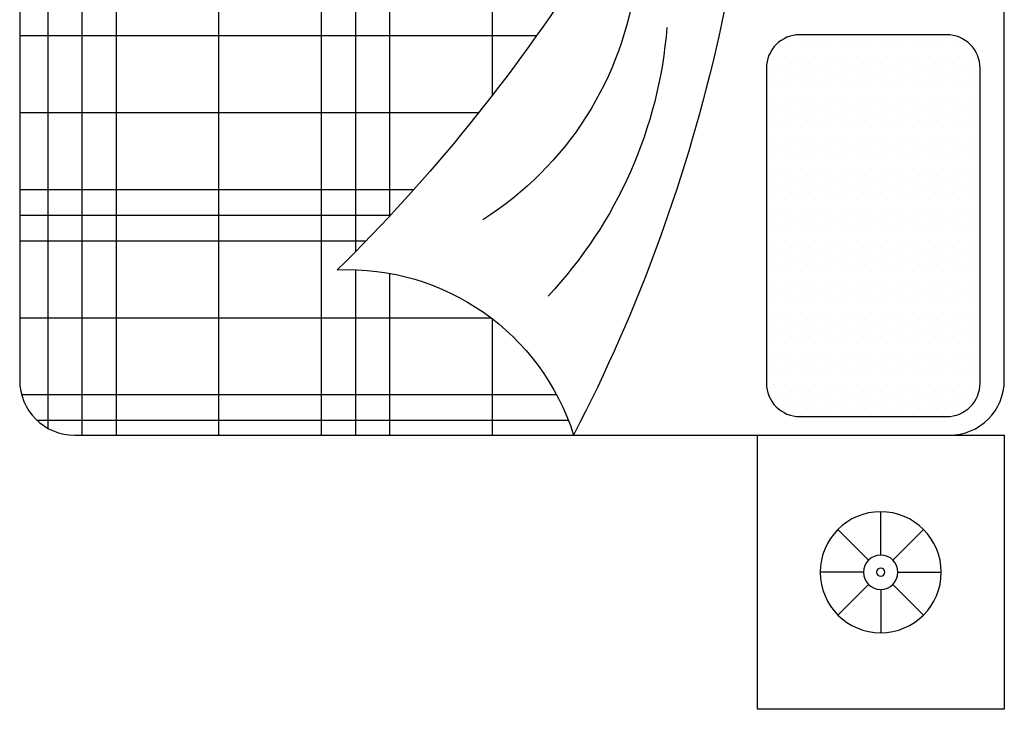
# Model space of a CAD drawing. Units: inches. Extents: x 528 to 2520, y -151 to 1354.
# Tile 38 of 41: x 2385 to 2440, y 731 to 770. Entities that reach past the tile are written whole.
import ezdxf

# ---------------------------------------------------------------- set-up
doc = ezdxf.new("R2010")
doc.units = ezdxf.units.IN
doc.header["$MEASUREMENT"] = 0
doc.layers.add('A-FURN', color=8, linetype='Continuous', lineweight=18)
doc.layers.add('BLOCK', color=6, linetype='Continuous')

# ---------------------------------------------------------------- blocks, each defined once
blk = doc.blocks.new('*X15')
at = {"color": 0}
for p, q in [((276.598, 451.25), (280.51, 451.25)), ((275.455, 450.625), (280.51, 450.625)), ((274.411, 450), (280.51, 450)), ((265.51, 448.125), (267.634, 448.125)), ((271.723, 448.125), (280.51, 448.125)), ((265.51, 446.25), (268.465, 446.25)), ((269.519, 446.25), (280.51, 446.25)), ((265.51, 445.625), (268.531, 445.625)), ((268.866, 445.625), (280.51, 445.625)), ((265.51, 445), (280.51, 445)), ((265.51, 443.125), (280.51, 443.125)), ((265.51, 441.25), (280.51, 441.25)), ((265.51, 440.625), (280.51, 440.625)), ((265.634, 440), (280.386, 440))]:
    blk.add_line(p, q, dxfattribs=at)
blk = doc.blocks.new('*X16')
at = {"color": 0}
for p, q in [((280.312, 439.886), (280.312, 452.896)), ((278.906, 439.482), (278.906, 452.338)), ((277.5, 439.482), (277.5, 451.702)), ((277.031, 439.482), (277.031, 451.471)), ((276.562, 439.482), (276.562, 451.231)), ((275.156, 439.482), (275.156, 450.451)), ((265.781, 439.797), (265.781, 449.511)), ((273.75, 439.482), (273.75, 449.576)), ((266.25, 439.517), (266.25, 449.296)), ((273.281, 439.482), (273.281, 449.261)), ((272.812, 439.482), (272.812, 448.934)), ((267.656, 439.482), (267.656, 448.095)), ((271.406, 439.482), (271.406, 447.876)), ((270, 439.482), (270, 446.689)), ((269.531, 439.482), (269.531, 446.262)), ((269.062, 439.482), (269.062, 445.817))]:
    blk.add_line(p, q, dxfattribs=at)
blk = doc.blocks.new('*X17')
at = {"color": 0}
for p, q in [((266.4375, 457.03125), (266.4375, 457.03125)), ((266.8125, 457.03125), (266.8125, 457.03125)), ((267.1875, 457.03125), (267.1875, 457.03125)), ((267.5625, 457.03125), (267.5625, 457.03125)), ((267.9375, 457.03125), (267.9375, 457.03125)), ((268.3125, 457.03125), (268.3125, 457.03125)), ((268.6875, 457.03125), (268.6875, 457.03125)), ((269.0625, 457.03125), (269.0625, 457.03125)), ((269.4375, 457.03125), (269.4375, 457.03125)), ((269.8125, 457.03125), (269.8125, 457.03125)), ((270.1875, 457.03125), (270.1875, 457.03125)), ((270.5625, 457.03125), (270.5625, 457.03125)), ((270.9375, 457.03125), (270.9375, 457.03125)), ((271.3125, 457.03125), (271.3125, 457.03125)), ((271.6875, 457.03125), (271.6875, 457.03125)), ((272.0625, 457.03125), (272.0625, 457.03125)), ((266.0625, 456.84375), (266.0625, 456.84375)), ((266.25, 456.9375), (266.25, 456.9375)), ((266.4375, 456.84375), (266.4375, 456.84375)), ((266.625, 456.9375), (266.625, 456.9375)), ((266.8125, 456.84375), (266.8125, 456.84375)), ((267, 456.9375), (267, 456.9375)), ((267.1875, 456.84375), (267.1875, 456.84375)), ((267.375, 456.9375), (267.375, 456.9375)), ((267.5625, 456.84375), (267.5625, 456.84375)), ((267.75, 456.9375), (267.75, 456.9375)), ((267.9375, 456.84375), (267.9375, 456.84375)), ((268.125, 456.9375), (268.125, 456.9375)), ((268.3125, 456.84375), (268.3125, 456.84375)), ((268.5, 456.9375), (268.5, 456.9375)), ((268.6875, 456.84375), (268.6875, 456.84375)), ((268.875, 456.9375), (268.875, 456.9375)), ((269.0625, 456.84375), (269.0625, 456.84375)), ((269.25, 456.9375), (269.25, 456.9375)), ((269.4375, 456.84375), (269.4375, 456.84375)), ((269.625, 456.9375), (269.625, 456.9375)), ((269.8125, 456.84375), (269.8125, 456.84375)), ((270, 456.9375), (270, 456.9375)), ((270.1875, 456.84375), (270.1875, 456.84375)), ((270.375, 456.9375), (270.375, 456.9375)), ((270.5625, 456.84375), (270.5625, 456.84375)), ((270.75, 456.9375), (270.75, 456.9375)), ((270.9375, 456.84375), (270.9375, 456.84375)), ((271.125, 456.9375), (271.125, 456.9375)), ((271.3125, 456.84375), (271.3125, 456.84375)), ((271.5, 456.9375), (271.5, 456.9375)), ((271.6875, 456.84375), (271.6875, 456.84375)), ((271.875, 456.9375), (271.875, 456.9375)), ((272.0625, 456.84375), (272.0625, 456.84375)), ((272.25, 456.9375), (272.25, 456.9375)), ((272.4375, 456.84375), (272.4375, 456.84375)), ((266.25, 456.75), (266.25, 456.75)), ((266.625, 456.75), (266.625, 456.75)), ((267, 456.75), (267, 456.75)), ((267.375, 456.75), (267.375, 456.75)), ((267.75, 456.75), (267.75, 456.75)), ((268.125, 456.75), (268.125, 456.75)), ((268.5, 456.75), (268.5, 456.75)), ((268.875, 456.75), (268.875, 456.75)), ((269.25, 456.75), (269.25, 456.75)), ((269.625, 456.75), (269.625, 456.75)), ((270, 456.75), (270, 456.75)), ((270.375, 456.75), (270.375, 456.75)), ((270.75, 456.75), (270.75, 456.75)), ((271.125, 456.75), (271.125, 456.75)), ((271.5, 456.75), (271.5, 456.75)), ((271.875, 456.75), (271.875, 456.75)), ((272.25, 456.75), (272.25, 456.75)), ((272.625, 456.75), (272.625, 456.75)), ((265.875, 456.5625), (265.875, 456.5625)), ((266.0625, 456.65625), (266.0625, 456.65625)), ((266.25, 456.5625), (266.25, 456.5625)), ((266.4375, 456.65625), (266.4375, 456.65625)), ((266.625, 456.5625), (266.625, 456.5625)), ((266.8125, 456.65625), (266.8125, 456.65625)), ((267, 456.5625), (267, 456.5625)), ((267.1875, 456.65625), (267.1875, 456.65625)), ((267.375, 456.5625), (267.375, 456.5625)), ((267.5625, 456.65625), (267.5625, 456.65625)), ((267.75, 456.5625), (267.75, 456.5625)), ((267.9375, 456.65625), (267.9375, 456.65625)), ((268.125, 456.5625), (268.125, 456.5625)), ((268.3125, 456.65625), (268.3125, 456.65625)), ((268.5, 456.5625), (268.5, 456.5625)), ((268.6875, 456.65625), (268.6875, 456.65625)), ((268.875, 456.5625), (268.875, 456.5625)), ((269.0625, 456.65625), (269.0625, 456.65625)), ((269.25, 456.5625), (269.25, 456.5625)), ((269.4375, 456.65625), (269.4375, 456.65625)), ((269.625, 456.5625), (269.625, 456.5625)), ((269.8125, 456.65625), (269.8125, 456.65625)), ((270, 456.5625), (270, 456.5625)), ((270.1875, 456.65625), (270.1875, 456.65625)), ((270.375, 456.5625), (270.375, 456.5625)), ((270.5625, 456.65625), (270.5625, 456.65625)), ((270.75, 456.5625), (270.75, 456.5625)), ((270.9375, 456.65625), (270.9375, 456.65625)), ((271.125, 456.5625), (271.125, 456.5625)), ((271.3125, 456.65625), (271.3125, 456.65625)), ((271.5, 456.5625), (271.5, 456.5625)), ((271.6875, 456.65625), (271.6875, 456.65625)), ((271.875, 456.5625), (271.875, 456.5625)), ((272.0625, 456.65625), (272.0625, 456.65625)), ((272.25, 456.5625), (272.25, 456.5625)), ((272.4375, 456.65625), (272.4375, 456.65625)), ((272.625, 456.5625), (272.625, 456.5625)), ((265.875, 456.375), (265.875, 456.375)), ((266.0625, 456.46875), (266.0625, 456.46875)), ((266.25, 456.375), (266.25, 456.375)), ((266.4375, 456.46875), (266.4375, 456.46875)), ((266.625, 456.375), (266.625, 456.375)), ((266.8125, 456.46875), (266.8125, 456.46875)), ((267, 456.375), (267, 456.375)), ((267.1875, 456.46875), (267.1875, 456.46875)), ((267.375, 456.375), (267.375, 456.375)), ((267.5625, 456.46875), (267.5625, 456.46875)), ((267.75, 456.375), (267.75, 456.375)), ((267.9375, 456.46875), (267.9375, 456.46875)), ((268.125, 456.375), (268.125, 456.375)), ((268.3125, 456.46875), (268.3125, 456.46875)), ((268.5, 456.375), (268.5, 456.375)), ((268.6875, 456.46875), (268.6875, 456.46875)), ((268.875, 456.375), (268.875, 456.375)), ((269.0625, 456.46875), (269.0625, 456.46875)), ((269.25, 456.375), (269.25, 456.375)), ((269.4375, 456.46875), (269.4375, 456.46875)), ((269.625, 456.375), (269.625, 456.375)), ((269.8125, 456.46875), (269.8125, 456.46875)), ((270, 456.375), (270, 456.375)), ((270.1875, 456.46875), (270.1875, 456.46875)), ((270.375, 456.375), (270.375, 456.375)), ((270.5625, 456.46875), (270.5625, 456.46875)), ((270.75, 456.375), (270.75, 456.375)), ((270.9375, 456.46875), (270.9375, 456.46875)), ((271.125, 456.375), (271.125, 456.375)), ((271.3125, 456.46875), (271.3125, 456.46875)), ((271.5, 456.375), (271.5, 456.375)), ((271.6875, 456.46875), (271.6875, 456.46875)), ((271.875, 456.375), (271.875, 456.375)), ((272.0625, 456.46875), (272.0625, 456.46875)), ((272.25, 456.375), (272.25, 456.375)), ((272.4375, 456.46875), (272.4375, 456.46875)), ((272.625, 456.375), (272.625, 456.375)), ((272.8125, 456.46875), (272.8125, 456.46875)), ((265.875, 456.1875), (265.875, 456.1875)), ((266.0625, 456.28125), (266.0625, 456.28125)), ((266.25, 456.1875), (266.25, 456.1875)), ((266.4375, 456.28125), (266.4375, 456.28125)), ((266.625, 456.1875), (266.625, 456.1875)), ((266.8125, 456.28125), (266.8125, 456.28125)), ((267, 456.1875), (267, 456.1875)), ((267.1875, 456.28125), (267.1875, 456.28125)), ((267.375, 456.1875), (267.375, 456.1875)), ((267.5625, 456.28125), (267.5625, 456.28125)), ((267.75, 456.1875), (267.75, 456.1875)), ((267.9375, 456.28125), (267.9375, 456.28125)), ((268.125, 456.1875), (268.125, 456.1875)), ((268.3125, 456.28125), (268.3125, 456.28125)), ((268.5, 456.1875), (268.5, 456.1875)), ((268.6875, 456.28125), (268.6875, 456.28125)), ((268.875, 456.1875), (268.875, 456.1875)), ((269.0625, 456.28125), (269.0625, 456.28125)), ((269.25, 456.1875), (269.25, 456.1875)), ((269.4375, 456.28125), (269.4375, 456.28125)), ((269.625, 456.1875), (269.625, 456.1875)), ((269.8125, 456.28125), (269.8125, 456.28125)), ((270, 456.1875), (270, 456.1875)), ((270.1875, 456.28125), (270.1875, 456.28125)), ((270.375, 456.1875), (270.375, 456.1875)), ((270.5625, 456.28125), (270.5625, 456.28125)), ((270.75, 456.1875), (270.75, 456.1875)), ((270.9375, 456.28125), (270.9375, 456.28125)), ((271.125, 456.1875), (271.125, 456.1875)), ((271.3125, 456.28125), (271.3125, 456.28125)), ((271.5, 456.1875), (271.5, 456.1875)), ((271.6875, 456.28125), (271.6875, 456.28125)), ((271.875, 456.1875), (271.875, 456.1875)), ((272.0625, 456.28125), (272.0625, 456.28125)), ((272.25, 456.1875), (272.25, 456.1875)), ((272.4375, 456.28125), (272.4375, 456.28125)), ((272.625, 456.1875), (272.625, 456.1875)), ((272.8125, 456.28125), (272.8125, 456.28125)), ((265.875, 456), (265.875, 456)), ((266.0625, 456.09375), (266.0625, 456.09375)), ((266.25, 456), (266.25, 456)), ((266.4375, 456.09375), (266.4375, 456.09375)), ((266.625, 456), (266.625, 456)), ((266.8125, 456.09375), (266.8125, 456.09375)), ((267, 456), (267, 456)), ((267.1875, 456.09375), (267.1875, 456.09375)), ((267.375, 456), (267.375, 456)), ((267.5625, 456.09375), (267.5625, 456.09375)), ((267.75, 456), (267.75, 456)), ((267.9375, 456.09375), (267.9375, 456.09375)), ((268.125, 456), (268.125, 456)), ((268.3125, 456.09375), (268.3125, 456.09375)), ((268.5, 456), (268.5, 456)), ((268.6875, 456.09375), (268.6875, 456.09375)), ((268.875, 456), (268.875, 456)), ((269.0625, 456.09375), (269.0625, 456.09375)), ((269.25, 456), (269.25, 456)), ((269.4375, 456.09375), (269.4375, 456.09375)), ((269.625, 456), (269.625, 456)), ((269.8125, 456.09375), (269.8125, 456.09375)), ((270, 456), (270, 456)), ((270.1875, 456.09375), (270.1875, 456.09375)), ((270.375, 456), (270.375, 456)), ((270.5625, 456.09375), (270.5625, 456.09375)), ((270.75, 456), (270.75, 456)), ((270.9375, 456.09375), (270.9375, 456.09375)), ((271.125, 456), (271.125, 456)), ((271.3125, 456.09375), (271.3125, 456.09375)), ((271.5, 456), (271.5, 456)), ((271.6875, 456.09375), (271.6875, 456.09375)), ((271.875, 456), (271.875, 456)), ((272.0625, 456.09375), (272.0625, 456.09375)), ((272.25, 456), (272.25, 456)), ((272.4375, 456.09375), (272.4375, 456.09375)), ((272.625, 456), (272.625, 456)), ((272.8125, 456.09375), (272.8125, 456.09375)), ((265.875, 455.8125), (265.875, 455.8125)), ((266.0625, 455.90625), (266.0625, 455.90625)), ((266.25, 455.8125), (266.25, 455.8125)), ((266.4375, 455.90625), (266.4375, 455.90625)), ((266.625, 455.8125), (266.625, 455.8125)), ((266.8125, 455.90625), (266.8125, 455.90625)), ((267, 455.8125), (267, 455.8125)), ((267.1875, 455.90625), (267.1875, 455.90625)), ((267.375, 455.8125), (267.375, 455.8125)), ((267.5625, 455.90625), (267.5625, 455.90625)), ((267.75, 455.8125), (267.75, 455.8125)), ((267.9375, 455.90625), (267.9375, 455.90625)), ((268.125, 455.8125), (268.125, 455.8125)), ((268.3125, 455.90625), (268.3125, 455.90625)), ((268.5, 455.8125), (268.5, 455.8125)), ((268.6875, 455.90625), (268.6875, 455.90625)), ((268.875, 455.8125), (268.875, 455.8125)), ((269.0625, 455.90625), (269.0625, 455.90625)), ((269.25, 455.8125), (269.25, 455.8125)), ((269.4375, 455.90625), (269.4375, 455.90625)), ((269.625, 455.8125), (269.625, 455.8125)), ((269.8125, 455.90625), (269.8125, 455.90625)), ((270, 455.8125), (270, 455.8125)), ((270.1875, 455.90625), (270.1875, 455.90625)), ((270.375, 455.8125), (270.375, 455.8125)), ((270.5625, 455.90625), (270.5625, 455.90625)), ((270.75, 455.8125), (270.75, 455.8125)), ((270.9375, 455.90625), (270.9375, 455.90625)), ((271.125, 455.8125), (271.125, 455.8125)), ((271.3125, 455.90625), (271.3125, 455.90625)), ((271.5, 455.8125), (271.5, 455.8125)), ((271.6875, 455.90625), (271.6875, 455.90625)), ((271.875, 455.8125), (271.875, 455.8125)), ((272.0625, 455.90625), (272.0625, 455.90625)), ((272.25, 455.8125), (272.25, 455.8125)), ((272.4375, 455.90625), (272.4375, 455.90625)), ((272.625, 455.8125), (272.625, 455.8125)), ((272.8125, 455.90625), (272.8125, 455.90625)), ((265.875, 455.625), (265.875, 455.625)), ((266.0625, 455.71875), (266.0625, 455.71875)), ((266.25, 455.625), (266.25, 455.625)), ((266.4375, 455.71875), (266.4375, 455.71875)), ((266.625, 455.625), (266.625, 455.625)), ((266.8125, 455.71875), (266.8125, 455.71875)), ((267, 455.625), (267, 455.625)), ((267.1875, 455.71875), (267.1875, 455.71875)), ((267.375, 455.625), (267.375, 455.625)), ((267.5625, 455.71875), (267.5625, 455.71875)), ((267.75, 455.625), (267.75, 455.625)), ((267.9375, 455.71875), (267.9375, 455.71875)), ((268.125, 455.625), (268.125, 455.625)), ((268.3125, 455.71875), (268.3125, 455.71875)), ((268.5, 455.625), (268.5, 455.625)), ((268.6875, 455.71875), (268.6875, 455.71875)), ((268.875, 455.625), (268.875, 455.625)), ((269.0625, 455.71875), (269.0625, 455.71875)), ((269.25, 455.625), (269.25, 455.625)), ((269.4375, 455.71875), (269.4375, 455.71875)), ((269.625, 455.625), (269.625, 455.625)), ((269.8125, 455.71875), (269.8125, 455.71875)), ((270, 455.625), (270, 455.625)), ((270.1875, 455.71875), (270.1875, 455.71875)), ((270.375, 455.625), (270.375, 455.625)), ((270.5625, 455.71875), (270.5625, 455.71875)), ((270.75, 455.625), (270.75, 455.625)), ((270.9375, 455.71875), (270.9375, 455.71875)), ((271.125, 455.625), (271.125, 455.625)), ((271.3125, 455.71875), (271.3125, 455.71875)), ((271.5, 455.625), (271.5, 455.625)), ((271.6875, 455.71875), (271.6875, 455.71875)), ((271.875, 455.625), (271.875, 455.625)), ((272.0625, 455.71875), (272.0625, 455.71875)), ((272.25, 455.625), (272.25, 455.625)), ((272.4375, 455.71875), (272.4375, 455.71875)), ((272.625, 455.625), (272.625, 455.625)), ((272.8125, 455.71875), (272.8125, 455.71875)), ((265.875, 455.4375), (265.875, 455.4375)), ((266.0625, 455.53125), (266.0625, 455.53125)), ((266.25, 455.4375), (266.25, 455.4375)), ((266.4375, 455.53125), (266.4375, 455.53125)), ((266.625, 455.4375), (266.625, 455.4375)), ((266.8125, 455.53125), (266.8125, 455.53125)), ((267, 455.4375), (267, 455.4375)), ((267.1875, 455.53125), (267.1875, 455.53125)), ((267.375, 455.4375), (267.375, 455.4375)), ((267.5625, 455.53125), (267.5625, 455.53125)), ((267.75, 455.4375), (267.75, 455.4375)), ((267.9375, 455.53125), (267.9375, 455.53125)), ((268.125, 455.4375), (268.125, 455.4375)), ((268.3125, 455.53125), (268.3125, 455.53125)), ((268.5, 455.4375), (268.5, 455.4375)), ((268.6875, 455.53125), (268.6875, 455.53125)), ((268.875, 455.4375), (268.875, 455.4375)), ((269.0625, 455.53125), (269.0625, 455.53125)), ((269.25, 455.4375), (269.25, 455.4375)), ((269.4375, 455.53125), (269.4375, 455.53125)), ((269.625, 455.4375), (269.625, 455.4375)), ((269.8125, 455.53125), (269.8125, 455.53125)), ((270, 455.4375), (270, 455.4375)), ((270.1875, 455.53125), (270.1875, 455.53125)), ((270.375, 455.4375), (270.375, 455.4375)), ((270.5625, 455.53125), (270.5625, 455.53125)), ((270.75, 455.4375), (270.75, 455.4375)), ((270.9375, 455.53125), (270.9375, 455.53125)), ((271.125, 455.4375), (271.125, 455.4375)), ((271.3125, 455.53125), (271.3125, 455.53125)), ((271.5, 455.4375), (271.5, 455.4375)), ((271.6875, 455.53125), (271.6875, 455.53125)), ((271.875, 455.4375), (271.875, 455.4375)), ((272.0625, 455.53125), (272.0625, 455.53125)), ((272.25, 455.4375), (272.25, 455.4375)), ((272.4375, 455.53125), (272.4375, 455.53125)), ((272.625, 455.4375), (272.625, 455.4375)), ((272.8125, 455.53125), (272.8125, 455.53125)), ((265.875, 455.25), (265.875, 455.25)), ((266.0625, 455.34375), (266.0625, 455.34375)), ((266.25, 455.25), (266.25, 455.25)), ((266.4375, 455.34375), (266.4375, 455.34375)), ((266.625, 455.25), (266.625, 455.25)), ((266.8125, 455.34375), (266.8125, 455.34375)), ((267, 455.25), (267, 455.25)), ((267.1875, 455.34375), (267.1875, 455.34375)), ((267.375, 455.25), (267.375, 455.25)), ((267.5625, 455.34375), (267.5625, 455.34375)), ((267.75, 455.25), (267.75, 455.25)), ((267.9375, 455.34375), (267.9375, 455.34375)), ((268.125, 455.25), (268.125, 455.25)), ((268.3125, 455.34375), (268.3125, 455.34375)), ((268.5, 455.25), (268.5, 455.25)), ((268.6875, 455.34375), (268.6875, 455.34375)), ((268.875, 455.25), (268.875, 455.25)), ((269.0625, 455.34375), (269.0625, 455.34375)), ((269.25, 455.25), (269.25, 455.25)), ((269.4375, 455.34375), (269.4375, 455.34375)), ((269.625, 455.25), (269.625, 455.25)), ((269.8125, 455.34375), (269.8125, 455.34375)), ((270, 455.25), (270, 455.25)), ((270.1875, 455.34375), (270.1875, 455.34375)), ((270.375, 455.25), (270.375, 455.25)), ((270.5625, 455.34375), (270.5625, 455.34375)), ((270.75, 455.25), (270.75, 455.25)), ((270.9375, 455.34375), (270.9375, 455.34375)), ((271.125, 455.25), (271.125, 455.25)), ((271.3125, 455.34375), (271.3125, 455.34375)), ((271.5, 455.25), (271.5, 455.25)), ((271.6875, 455.34375), (271.6875, 455.34375)), ((271.875, 455.25), (271.875, 455.25)), ((272.0625, 455.34375), (272.0625, 455.34375)), ((272.25, 455.25), (272.25, 455.25)), ((272.4375, 455.34375), (272.4375, 455.34375)), ((272.625, 455.25), (272.625, 455.25)), ((272.8125, 455.34375), (272.8125, 455.34375)), ((265.875, 455.0625), (265.875, 455.0625)), ((266.0625, 455.15625), (266.0625, 455.15625)), ((266.25, 455.0625), (266.25, 455.0625)), ((266.4375, 455.15625), (266.4375, 455.15625)), ((266.625, 455.0625), (266.625, 455.0625)), ((266.8125, 455.15625), (266.8125, 455.15625)), ((267, 455.0625), (267, 455.0625)), ((267.1875, 455.15625), (267.1875, 455.15625)), ((267.375, 455.0625), (267.375, 455.0625)), ((267.5625, 455.15625), (267.5625, 455.15625)), ((267.75, 455.0625), (267.75, 455.0625)), ((267.9375, 455.15625), (267.9375, 455.15625)), ((268.125, 455.0625), (268.125, 455.0625)), ((268.3125, 455.15625), (268.3125, 455.15625)), ((268.5, 455.0625), (268.5, 455.0625)), ((268.6875, 455.15625), (268.6875, 455.15625)), ((268.875, 455.0625), (268.875, 455.0625)), ((269.0625, 455.15625), (269.0625, 455.15625)), ((269.25, 455.0625), (269.25, 455.0625)), ((269.4375, 455.15625), (269.4375, 455.15625)), ((269.625, 455.0625), (269.625, 455.0625)), ((269.8125, 455.15625), (269.8125, 455.15625)), ((270, 455.0625), (270, 455.0625)), ((270.1875, 455.15625), (270.1875, 455.15625)), ((270.375, 455.0625), (270.375, 455.0625)), ((270.5625, 455.15625), (270.5625, 455.15625)), ((270.75, 455.0625), (270.75, 455.0625)), ((270.9375, 455.15625), (270.9375, 455.15625)), ((271.125, 455.0625), (271.125, 455.0625)), ((271.3125, 455.15625), (271.3125, 455.15625)), ((271.5, 455.0625), (271.5, 455.0625)), ((271.6875, 455.15625), (271.6875, 455.15625)), ((271.875, 455.0625), (271.875, 455.0625)), ((272.0625, 455.15625), (272.0625, 455.15625)), ((272.25, 455.0625), (272.25, 455.0625)), ((272.4375, 455.15625), (272.4375, 455.15625)), ((272.625, 455.0625), (272.625, 455.0625)), ((272.8125, 455.15625), (272.8125, 455.15625)), ((265.875, 454.875), (265.875, 454.875)), ((266.0625, 454.96875), (266.0625, 454.96875)), ((266.25, 454.875), (266.25, 454.875)), ((266.4375, 454.96875), (266.4375, 454.96875)), ((266.625, 454.875), (266.625, 454.875)), ((266.8125, 454.96875), (266.8125, 454.96875)), ((267, 454.875), (267, 454.875)), ((267.1875, 454.96875), (267.1875, 454.96875)), ((267.375, 454.875), (267.375, 454.875)), ((267.5625, 454.96875), (267.5625, 454.96875)), ((267.75, 454.875), (267.75, 454.875)), ((267.9375, 454.96875), (267.9375, 454.96875)), ((268.125, 454.875), (268.125, 454.875)), ((268.3125, 454.96875), (268.3125, 454.96875)), ((268.5, 454.875), (268.5, 454.875)), ((268.6875, 454.96875), (268.6875, 454.96875)), ((268.875, 454.875), (268.875, 454.875)), ((269.0625, 454.96875), (269.0625, 454.96875)), ((269.25, 454.875), (269.25, 454.875)), ((269.4375, 454.96875), (269.4375, 454.96875)), ((269.625, 454.875), (269.625, 454.875)), ((269.8125, 454.96875), (269.8125, 454.96875)), ((270, 454.875), (270, 454.875)), ((270.1875, 454.96875), (270.1875, 454.96875)), ((270.375, 454.875), (270.375, 454.875)), ((270.5625, 454.96875), (270.5625, 454.96875)), ((270.75, 454.875), (270.75, 454.875)), ((270.9375, 454.96875), (270.9375, 454.96875)), ((271.125, 454.875), (271.125, 454.875)), ((271.3125, 454.96875), (271.3125, 454.96875)), ((271.5, 454.875), (271.5, 454.875)), ((271.6875, 454.96875), (271.6875, 454.96875)), ((271.875, 454.875), (271.875, 454.875)), ((272.0625, 454.96875), (272.0625, 454.96875)), ((272.25, 454.875), (272.25, 454.875)), ((272.4375, 454.96875), (272.4375, 454.96875)), ((272.625, 454.875), (272.625, 454.875)), ((272.8125, 454.96875), (272.8125, 454.96875)), ((265.875, 454.6875), (265.875, 454.6875)), ((266.0625, 454.78125), (266.0625, 454.78125)), ((266.25, 454.6875), (266.25, 454.6875)), ((266.4375, 454.78125), (266.4375, 454.78125)), ((266.625, 454.6875), (266.625, 454.6875)), ((266.8125, 454.78125), (266.8125, 454.78125)), ((267, 454.6875), (267, 454.6875)), ((267.1875, 454.78125), (267.1875, 454.78125)), ((267.375, 454.6875), (267.375, 454.6875)), ((267.5625, 454.78125), (267.5625, 454.78125)), ((267.75, 454.6875), (267.75, 454.6875)), ((267.9375, 454.78125), (267.9375, 454.78125)), ((268.125, 454.6875), (268.125, 454.6875)), ((268.3125, 454.78125), (268.3125, 454.78125)), ((268.5, 454.6875), (268.5, 454.6875)), ((268.6875, 454.78125), (268.6875, 454.78125)), ((268.875, 454.6875), (268.875, 454.6875)), ((269.0625, 454.78125), (269.0625, 454.78125)), ((269.25, 454.6875), (269.25, 454.6875)), ((269.4375, 454.78125), (269.4375, 454.78125)), ((269.625, 454.6875), (269.625, 454.6875)), ((269.8125, 454.78125), (269.8125, 454.78125)), ((270, 454.6875), (270, 454.6875)), ((270.1875, 454.78125), (270.1875, 454.78125)), ((270.375, 454.6875), (270.375, 454.6875)), ((270.5625, 454.78125), (270.5625, 454.78125)), ((270.75, 454.6875), (270.75, 454.6875)), ((270.9375, 454.78125), (270.9375, 454.78125)), ((271.125, 454.6875), (271.125, 454.6875)), ((271.3125, 454.78125), (271.3125, 454.78125)), ((271.5, 454.6875), (271.5, 454.6875)), ((271.6875, 454.78125), (271.6875, 454.78125)), ((271.875, 454.6875), (271.875, 454.6875)), ((272.0625, 454.78125), (272.0625, 454.78125)), ((272.25, 454.6875), (272.25, 454.6875)), ((272.4375, 454.78125), (272.4375, 454.78125)), ((272.625, 454.6875), (272.625, 454.6875)), ((272.8125, 454.78125), (272.8125, 454.78125)), ((266.0625, 454.59375), (266.0625, 454.59375)), ((266.4375, 454.59375), (266.4375, 454.59375)), ((266.8125, 454.59375), (266.8125, 454.59375)), ((267.1875, 454.59375), (267.1875, 454.59375)), ((267.5625, 454.59375), (267.5625, 454.59375)), ((267.9375, 454.59375), (267.9375, 454.59375)), ((268.3125, 454.59375), (268.3125, 454.59375)), ((268.6875, 454.59375), (268.6875, 454.59375)), ((269.0625, 454.59375), (269.0625, 454.59375)), ((269.4375, 454.59375), (269.4375, 454.59375)), ((269.8125, 454.59375), (269.8125, 454.59375)), ((270.1875, 454.59375), (270.1875, 454.59375)), ((270.5625, 454.59375), (270.5625, 454.59375)), ((270.9375, 454.59375), (270.9375, 454.59375)), ((271.3125, 454.59375), (271.3125, 454.59375)), ((271.6875, 454.59375), (271.6875, 454.59375)), ((272.0625, 454.59375), (272.0625, 454.59375)), ((272.4375, 454.59375), (272.4375, 454.59375)), ((272.8125, 454.59375), (272.8125, 454.59375)), ((265.875, 454.5), (265.875, 454.5)), ((266.0625, 454.40625), (266.0625, 454.40625)), ((266.25, 454.5), (266.25, 454.5)), ((266.4375, 454.40625), (266.4375, 454.40625)), ((266.625, 454.5), (266.625, 454.5)), ((266.8125, 454.40625), (266.8125, 454.40625)), ((267, 454.5), (267, 454.5)), ((267.1875, 454.40625), (267.1875, 454.40625)), ((267.375, 454.5), (267.375, 454.5)), ((267.5625, 454.40625), (267.5625, 454.40625)), ((267.75, 454.5), (267.75, 454.5)), ((267.9375, 454.40625), (267.9375, 454.40625)), ((268.125, 454.5), (268.125, 454.5)), ((268.3125, 454.40625), (268.3125, 454.40625)), ((268.5, 454.5), (268.5, 454.5)), ((268.6875, 454.40625), (268.6875, 454.40625)), ((268.875, 454.5), (268.875, 454.5)), ((269.0625, 454.40625), (269.0625, 454.40625)), ((269.25, 454.5), (269.25, 454.5)), ((269.4375, 454.40625), (269.4375, 454.40625)), ((269.625, 454.5), (269.625, 454.5)), ((269.8125, 454.40625), (269.8125, 454.40625)), ((270, 454.5), (270, 454.5)), ((270.1875, 454.40625), (270.1875, 454.40625)), ((270.375, 454.5), (270.375, 454.5)), ((270.5625, 454.40625), (270.5625, 454.40625)), ((270.75, 454.5), (270.75, 454.5)), ((270.9375, 454.40625), (270.9375, 454.40625)), ((271.125, 454.5), (271.125, 454.5)), ((271.3125, 454.40625), (271.3125, 454.40625)), ((271.5, 454.5), (271.5, 454.5)), ((271.6875, 454.40625), (271.6875, 454.40625)), ((271.875, 454.5), (271.875, 454.5)), ((272.0625, 454.40625), (272.0625, 454.40625)), ((272.25, 454.5), (272.25, 454.5)), ((272.4375, 454.40625), (272.4375, 454.40625)), ((272.625, 454.5), (272.625, 454.5)), ((272.8125, 454.40625), (272.8125, 454.40625)), ((265.875, 454.3125), (265.875, 454.3125)), ((266.0625, 454.21875), (266.0625, 454.21875)), ((266.25, 454.3125), (266.25, 454.3125)), ((266.4375, 454.21875), (266.4375, 454.21875)), ((266.625, 454.3125), (266.625, 454.3125)), ((266.8125, 454.21875), (266.8125, 454.21875)), ((267, 454.3125), (267, 454.3125)), ((267.1875, 454.21875), (267.1875, 454.21875)), ((267.375, 454.3125), (267.375, 454.3125)), ((267.5625, 454.21875), (267.5625, 454.21875)), ((267.75, 454.3125), (267.75, 454.3125)), ((267.9375, 454.21875), (267.9375, 454.21875)), ((268.125, 454.3125), (268.125, 454.3125)), ((268.3125, 454.21875), (268.3125, 454.21875)), ((268.5, 454.3125), (268.5, 454.3125)), ((268.6875, 454.21875), (268.6875, 454.21875)), ((268.875, 454.3125), (268.875, 454.3125)), ((269.0625, 454.21875), (269.0625, 454.21875)), ((269.25, 454.3125), (269.25, 454.3125)), ((269.4375, 454.21875), (269.4375, 454.21875)), ((269.625, 454.3125), (269.625, 454.3125)), ((269.8125, 454.21875), (269.8125, 454.21875)), ((270, 454.3125), (270, 454.3125)), ((270.1875, 454.21875), (270.1875, 454.21875)), ((270.375, 454.3125), (270.375, 454.3125)), ((270.5625, 454.21875), (270.5625, 454.21875)), ((270.75, 454.3125), (270.75, 454.3125)), ((270.9375, 454.21875), (270.9375, 454.21875)), ((271.125, 454.3125), (271.125, 454.3125)), ((271.3125, 454.21875), (271.3125, 454.21875)), ((271.5, 454.3125), (271.5, 454.3125)), ((271.6875, 454.21875), (271.6875, 454.21875)), ((271.875, 454.3125), (271.875, 454.3125)), ((272.0625, 454.21875), (272.0625, 454.21875)), ((272.25, 454.3125), (272.25, 454.3125)), ((272.4375, 454.21875), (272.4375, 454.21875)), ((272.625, 454.3125), (272.625, 454.3125)), ((272.8125, 454.21875), (272.8125, 454.21875)), ((265.875, 454.125), (265.875, 454.125)), ((266.0625, 454.03125), (266.0625, 454.03125)), ((266.25, 454.125), (266.25, 454.125)), ((266.4375, 454.03125), (266.4375, 454.03125)), ((266.625, 454.125), (266.625, 454.125)), ((266.8125, 454.03125), (266.8125, 454.03125)), ((267, 454.125), (267, 454.125)), ((267.1875, 454.03125), (267.1875, 454.03125)), ((267.375, 454.125), (267.375, 454.125)), ((267.5625, 454.03125), (267.5625, 454.03125)), ((267.75, 454.125), (267.75, 454.125)), ((267.9375, 454.03125), (267.9375, 454.03125)), ((268.125, 454.125), (268.125, 454.125)), ((268.3125, 454.03125), (268.3125, 454.03125)), ((268.5, 454.125), (268.5, 454.125)), ((268.6875, 454.03125), (268.6875, 454.03125)), ((268.875, 454.125), (268.875, 454.125)), ((269.0625, 454.03125), (269.0625, 454.03125)), ((269.25, 454.125), (269.25, 454.125)), ((269.4375, 454.03125), (269.4375, 454.03125)), ((269.625, 454.125), (269.625, 454.125)), ((269.8125, 454.03125), (269.8125, 454.03125)), ((270, 454.125), (270, 454.125)), ((270.1875, 454.03125), (270.1875, 454.03125)), ((270.375, 454.125), (270.375, 454.125)), ((270.5625, 454.03125), (270.5625, 454.03125)), ((270.75, 454.125), (270.75, 454.125)), ((270.9375, 454.03125), (270.9375, 454.03125)), ((271.125, 454.125), (271.125, 454.125)), ((271.3125, 454.03125), (271.3125, 454.03125)), ((271.5, 454.125), (271.5, 454.125)), ((271.6875, 454.03125), (271.6875, 454.03125)), ((271.875, 454.125), (271.875, 454.125)), ((272.0625, 454.03125), (272.0625, 454.03125)), ((272.25, 454.125), (272.25, 454.125)), ((272.4375, 454.03125), (272.4375, 454.03125)), ((272.625, 454.125), (272.625, 454.125)), ((272.8125, 454.03125), (272.8125, 454.03125)), ((265.875, 453.9375), (265.875, 453.9375)), ((266.0625, 453.84375), (266.0625, 453.84375)), ((266.25, 453.9375), (266.25, 453.9375)), ((266.4375, 453.84375), (266.4375, 453.84375)), ((266.625, 453.9375), (266.625, 453.9375)), ((266.8125, 453.84375), (266.8125, 453.84375)), ((267, 453.9375), (267, 453.9375)), ((267.1875, 453.84375), (267.1875, 453.84375)), ((267.375, 453.9375), (267.375, 453.9375)), ((267.5625, 453.84375), (267.5625, 453.84375)), ((267.75, 453.9375), (267.75, 453.9375)), ((267.9375, 453.84375), (267.9375, 453.84375)), ((268.125, 453.9375), (268.125, 453.9375)), ((268.3125, 453.84375), (268.3125, 453.84375)), ((268.5, 453.9375), (268.5, 453.9375)), ((268.6875, 453.84375), (268.6875, 453.84375)), ((268.875, 453.9375), (268.875, 453.9375)), ((269.0625, 453.84375), (269.0625, 453.84375)), ((269.25, 453.9375), (269.25, 453.9375)), ((269.4375, 453.84375), (269.4375, 453.84375)), ((269.625, 453.9375), (269.625, 453.9375)), ((269.8125, 453.84375), (269.8125, 453.84375)), ((270, 453.9375), (270, 453.9375)), ((270.1875, 453.84375), (270.1875, 453.84375)), ((270.375, 453.9375), (270.375, 453.9375)), ((270.5625, 453.84375), (270.5625, 453.84375)), ((270.75, 453.9375), (270.75, 453.9375)), ((270.9375, 453.84375), (270.9375, 453.84375)), ((271.125, 453.9375), (271.125, 453.9375)), ((271.3125, 453.84375), (271.3125, 453.84375)), ((271.5, 453.9375), (271.5, 453.9375)), ((271.6875, 453.84375), (271.6875, 453.84375)), ((271.875, 453.9375), (271.875, 453.9375)), ((272.0625, 453.84375), (272.0625, 453.84375)), ((272.25, 453.9375), (272.25, 453.9375)), ((272.4375, 453.84375), (272.4375, 453.84375)), ((272.625, 453.9375), (272.625, 453.9375)), ((272.8125, 453.84375), (272.8125, 453.84375)), ((265.875, 453.75), (265.875, 453.75)), ((266.0625, 453.65625), (266.0625, 453.65625)), ((266.25, 453.75), (266.25, 453.75)), ((266.4375, 453.65625), (266.4375, 453.65625)), ((266.625, 453.75), (266.625, 453.75)), ((266.8125, 453.65625), (266.8125, 453.65625)), ((267, 453.75), (267, 453.75)), ((267.1875, 453.65625), (267.1875, 453.65625)), ((267.375, 453.75), (267.375, 453.75)), ((267.5625, 453.65625), (267.5625, 453.65625)), ((267.75, 453.75), (267.75, 453.75)), ((267.9375, 453.65625), (267.9375, 453.65625)), ((268.125, 453.75), (268.125, 453.75)), ((268.3125, 453.65625), (268.3125, 453.65625)), ((268.5, 453.75), (268.5, 453.75)), ((268.6875, 453.65625), (268.6875, 453.65625)), ((268.875, 453.75), (268.875, 453.75)), ((269.0625, 453.65625), (269.0625, 453.65625)), ((269.25, 453.75), (269.25, 453.75)), ((269.4375, 453.65625), (269.4375, 453.65625)), ((269.625, 453.75), (269.625, 453.75)), ((269.8125, 453.65625), (269.8125, 453.65625)), ((270, 453.75), (270, 453.75)), ((270.1875, 453.65625), (270.1875, 453.65625)), ((270.375, 453.75), (270.375, 453.75)), ((270.5625, 453.65625), (270.5625, 453.65625)), ((270.75, 453.75), (270.75, 453.75)), ((270.9375, 453.65625), (270.9375, 453.65625)), ((271.125, 453.75), (271.125, 453.75)), ((271.3125, 453.65625), (271.3125, 453.65625)), ((271.5, 453.75), (271.5, 453.75)), ((271.6875, 453.65625), (271.6875, 453.65625)), ((271.875, 453.75), (271.875, 453.75)), ((272.0625, 453.65625), (272.0625, 453.65625)), ((272.25, 453.75), (272.25, 453.75)), ((272.4375, 453.65625), (272.4375, 453.65625)), ((272.625, 453.75), (272.625, 453.75)), ((272.8125, 453.65625), (272.8125, 453.65625)), ((266.0625, 453.46875), (266.0625, 453.46875)), ((266.25, 453.5625), (266.25, 453.5625)), ((266.4375, 453.46875), (266.4375, 453.46875)), ((266.625, 453.5625), (266.625, 453.5625)), ((266.8125, 453.46875), (266.8125, 453.46875)), ((267, 453.5625), (267, 453.5625)), ((267.1875, 453.46875), (267.1875, 453.46875)), ((267.375, 453.5625), (267.375, 453.5625)), ((267.5625, 453.46875), (267.5625, 453.46875)), ((267.75, 453.5625), (267.75, 453.5625)), ((267.9375, 453.46875), (267.9375, 453.46875)), ((268.125, 453.5625), (268.125, 453.5625)), ((268.3125, 453.46875), (268.3125, 453.46875)), ((268.5, 453.5625), (268.5, 453.5625)), ((268.6875, 453.46875), (268.6875, 453.46875)), ((268.875, 453.5625), (268.875, 453.5625)), ((269.0625, 453.46875), (269.0625, 453.46875)), ((269.25, 453.5625), (269.25, 453.5625)), ((269.4375, 453.46875), (269.4375, 453.46875)), ((269.625, 453.5625), (269.625, 453.5625)), ((269.8125, 453.46875), (269.8125, 453.46875)), ((270, 453.5625), (270, 453.5625)), ((270.1875, 453.46875), (270.1875, 453.46875)), ((270.375, 453.5625), (270.375, 453.5625)), ((270.5625, 453.46875), (270.5625, 453.46875)), ((270.75, 453.5625), (270.75, 453.5625)), ((270.9375, 453.46875), (270.9375, 453.46875)), ((271.125, 453.5625), (271.125, 453.5625)), ((271.3125, 453.46875), (271.3125, 453.46875)), ((271.5, 453.5625), (271.5, 453.5625)), ((271.6875, 453.46875), (271.6875, 453.46875)), ((271.875, 453.5625), (271.875, 453.5625)), ((272.0625, 453.46875), (272.0625, 453.46875)), ((272.25, 453.5625), (272.25, 453.5625)), ((272.4375, 453.46875), (272.4375, 453.46875)), ((272.625, 453.5625), (272.625, 453.5625)), ((266.0625, 453.28125), (266.0625, 453.28125)), ((266.25, 453.375), (266.25, 453.375)), ((266.4375, 453.28125), (266.4375, 453.28125)), ((266.625, 453.375), (266.625, 453.375)), ((266.8125, 453.28125), (266.8125, 453.28125)), ((267, 453.375), (267, 453.375)), ((267.1875, 453.28125), (267.1875, 453.28125)), ((267.375, 453.375), (267.375, 453.375)), ((267.5625, 453.28125), (267.5625, 453.28125)), ((267.75, 453.375), (267.75, 453.375)), ((267.9375, 453.28125), (267.9375, 453.28125)), ((268.125, 453.375), (268.125, 453.375)), ((268.3125, 453.28125), (268.3125, 453.28125)), ((268.5, 453.375), (268.5, 453.375)), ((268.6875, 453.28125), (268.6875, 453.28125)), ((268.875, 453.375), (268.875, 453.375)), ((269.0625, 453.28125), (269.0625, 453.28125)), ((269.25, 453.375), (269.25, 453.375)), ((269.4375, 453.28125), (269.4375, 453.28125)), ((269.625, 453.375), (269.625, 453.375)), ((269.8125, 453.28125), (269.8125, 453.28125)), ((270, 453.375), (270, 453.375)), ((270.1875, 453.28125), (270.1875, 453.28125)), ((270.375, 453.375), (270.375, 453.375)), ((270.5625, 453.28125), (270.5625, 453.28125)), ((270.75, 453.375), (270.75, 453.375)), ((270.9375, 453.28125), (270.9375, 453.28125)), ((271.125, 453.375), (271.125, 453.375)), ((271.3125, 453.28125), (271.3125, 453.28125)), ((271.5, 453.375), (271.5, 453.375)), ((271.6875, 453.28125), (271.6875, 453.28125)), ((271.875, 453.375), (271.875, 453.375)), ((272.0625, 453.28125), (272.0625, 453.28125)), ((272.25, 453.375), (272.25, 453.375)), ((272.4375, 453.28125), (272.4375, 453.28125)), ((272.625, 453.375), (272.625, 453.375)), ((266.25, 453.1875), (266.25, 453.1875)), ((266.625, 453.1875), (266.625, 453.1875)), ((267, 453.1875), (267, 453.1875)), ((267.375, 453.1875), (267.375, 453.1875)), ((267.75, 453.1875), (267.75, 453.1875)), ((268.125, 453.1875), (268.125, 453.1875)), ((268.5, 453.1875), (268.5, 453.1875)), ((268.875, 453.1875), (268.875, 453.1875)), ((269.25, 453.1875), (269.25, 453.1875)), ((269.625, 453.1875), (269.625, 453.1875)), ((270, 453.1875), (270, 453.1875)), ((270.375, 453.1875), (270.375, 453.1875)), ((270.75, 453.1875), (270.75, 453.1875)), ((271.125, 453.1875), (271.125, 453.1875)), ((271.5, 453.1875), (271.5, 453.1875)), ((271.875, 453.1875), (271.875, 453.1875)), ((272.25, 453.1875), (272.25, 453.1875))]:
    blk.add_line(p, q, dxfattribs=at)
blk = doc.blocks.new('A$C52E67D0D')
at = {"layer": 'BLOCK'}
for p, q in [((250.5, 1605.5), (250.5, 1684.7)), ((228.3, 1596.3), (172.3, 1652.3)), ((272.7, 1596.3), (328.7, 1652.3)), ((219.1, 1574.1), (139.9, 1574.1)), ((281.9, 1574.1), (361.1, 1574.1)), ((228.3, 1551.9), (172.3, 1495.9)), ((272.7, 1551.9), (328.7, 1495.9)), ((250.5, 1542.8), (250.5, 1463.5))]:
    blk.add_line(p, q, dxfattribs=at)
for points in [[(1901, 0), (601, 0, -0.414214), (501, 100), (501, 1700, -0.414214), (601, 1800), (1901, 1800, -0.414214), (2001, 1700), (2001, 100, -0.414214)], [(1171.8, 1365.1), (595.8, 1365.1, -0.414214), (535, 1425.9), (535, 1694.8, -0.414214), (595.8, 1755.7), (1171.8, 1755.7, -0.414214), (1232.6, 1694.8), (1232.6, 1425.9, -0.414214)]]:
    blk.add_lwpolyline(points, format="xyb", close=True, dxfattribs=at)
blk.add_lwpolyline([(501, 1348.6), (501, 1799.6), (0, 1799.6), (0, 1348.6)], close=True, dxfattribs=at)
for radius in [110.6, 31.4, 7.46]:
    blk.add_circle((250.5, 1574.1), radius, dxfattribs=at)
for centre, radius, start, end in [((1888.6, -1664.5), 3015.3, 87.8642, 117.4001), ((3101, -1685.8), 3227.7, 109.926, 135.3977), ((1308.8, 377.9), 807.6, 94.4436, 133.2788), ((1410.8, 520.2), 610.8, 97.2157, 147.6656), ((371.4, 600.4), 432, 357.3792, 72.5379)]:
    blk.add_arc(centre, radius, start, end, dxfattribs=at)
at = {"layer": 'BLOCK', "xscale": 100, "yscale": 100, "zscale": 100}
for name in ['*X17', '*X16', '*X15']:
    blk.add_blockref(name, (-26050, -43948.2), dxfattribs=at)

msp = doc.modelspace()

# ---------------------------------------------------------------- block references
at = {"layer": 'A-FURN', "xscale": -0.0306954436450662, "yscale": 0.0306954436450662, "zscale": 0.0306954436450662, "rotation": 270}
msp.add_blockref('A$C52E67D0D', (2385.117, 731.467), dxfattribs=at)

doc.saveas('drawing.dxf')
